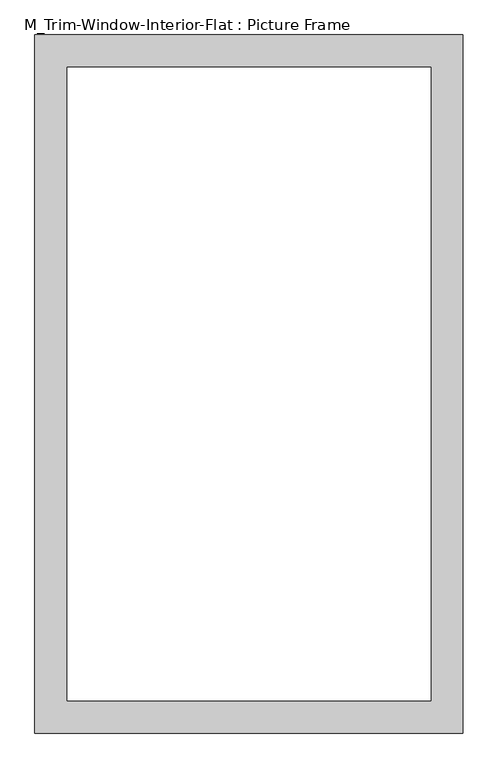
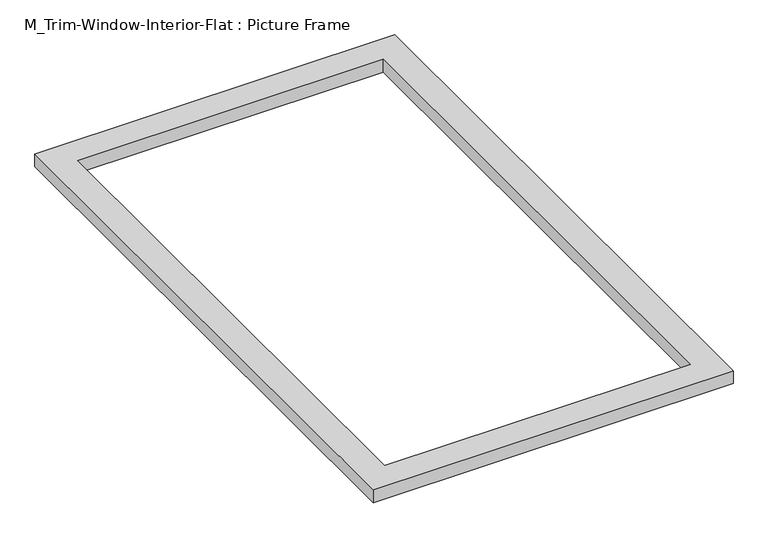
"""IFC4 building model written with IfcOpenShell, lengths in millimetres: proxy geometry, M_Trim-Window-Interior-Flat : Picture Frame."""

from ifc_helpers import new_model, si_unit, origin, origin_with_axes, place, context, project, spatial, polyline, outline, extrude, source, transform, mapped, element, save


def m_trim_window_interior_flat_picture_frame_c294611c(model_context):
    return source(origin(), model_context, "Body", "SweptSolid", [
        extrude(outline(polyline([(397.3, 47.3), (397.3, -1247.3), (-397.3, -1247.3), (-397.3, 47.3), (397.3, 47.3)]), holes=[polyline([(337.3, -12.7), (-337.3, -12.7), (-337.3, -1187.3), (337.3, -1187.3), (337.3, -12.7)])]), origin_with_axes(), (0.0, 0.0, 1.0), 30.0),
    ])


if __name__ == "__main__":
    model = new_model("IFC4")
    model_context = context("Model", 3, world=origin())
    ifc_project = project(units=[si_unit("LENGTHUNIT", "METRE", prefix="MILLI")], contexts=[model_context])
    site = spatial("IfcSite", under=ifc_project)
    building = spatial("IfcBuilding", under=site)
    placement = place(None, origin())
    m_trim_window_interior_flat_picture_frame_shape = m_trim_window_interior_flat_picture_frame_c294611c(model_context)
    element("IfcBuildingElementProxy", 1, Name="M_Trim-Window-Interior-Flat : Picture Frame", ObjectType="M_Trim-Window-Interior-Flat : Picture Frame", at=placement, inside=building, context=model_context, shape_type="MappedRepresentation", body=[
        mapped(m_trim_window_interior_flat_picture_frame_shape, transform((0.0, 0.0, 0.0), x_axis=(1.0, 0.0, 0.0), y_axis=(0.0, 1.0, 0.0), z_axis=(0.0, 0.0, 1.0))),
    ])
    save(model, "model.ifc")

# Revit data of these elements
# Type "M_Trim-Window-Interior-Flat : Picture Frame"
#   Trim Thickness_Picture Frame = 30 mm
#   Trim Width = 60 mm
#   Trim Thickness_with Sill = 20 mm
#   Sill Thickness = 30 mm
#   Opening Width [instance default] = 600 mm
#   Opening Height [instance default] = 900 mm
#   Default Elevation = 1200 mm
#   Sill = no
#   Picture Frame = yes
#   Trim Material [instance default] = none
# Element 1 (IfcBuildingElementProxy, "M_Trim-Window-Interior-Flat : Picture Frame")
#   Opening Width = 700 mm
#   Opening Height = 1200 mm
#   Trim Material = Wood - Stained
#   Materials on its faces: "Wood - Stained"
# Materials
#   "Wood - Stained": class "Wood", colour RGB 173 132 96, transparency 0, Cost = 0
